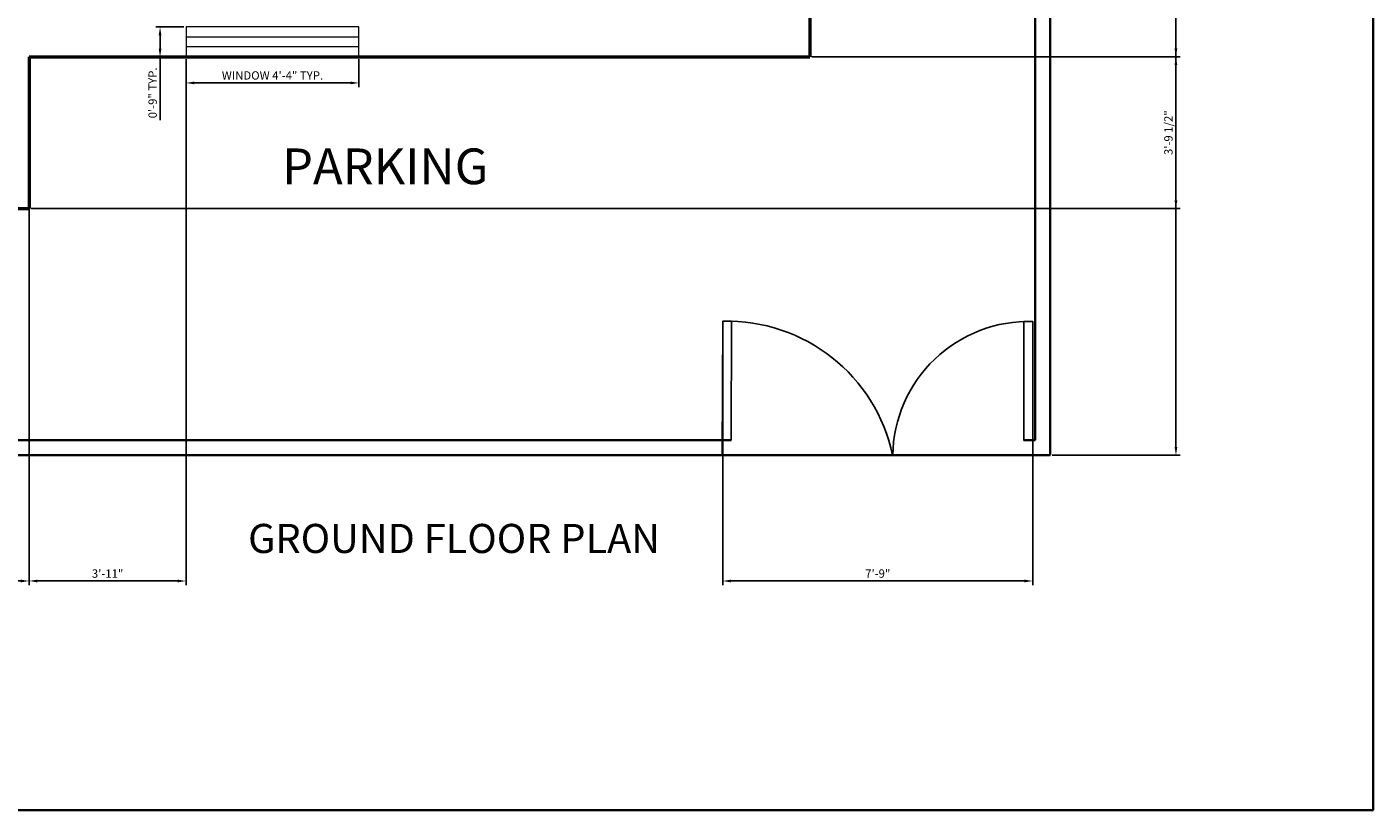
# Model space of a CAD drawing. Units: inches. Extents: x 65 to 818, y -87 to 880.
# Tile 3 of 6: x 414 to 818, y -87 to 148. Entities that reach past the tile are written whole.
import ezdxf

# ---------------------------------------------------------------- set-up
doc = ezdxf.new("R2010")
doc.units = ezdxf.units.IN
for name, color, linetype, lineweight in [('A-ANNO-DIMS', 2, 'Continuous', 18), ('A-ANNO-TEXT', 7, 'Continuous', 25), ('A-ANNO-TTLB', 7, 'Continuous', 35), ('A-AREA-IDEN', 7, 'Continuous', 25), ('A-GLAZ', 4, 'Continuous', 18), ('A-WALL', 7, 'Continuous', 50), ('C-PROP', 7, 'Continuous', 35), ('L-SITE-GATE', 3, 'Continuous', 25)]:
    doc.layers.add(name, color=color, linetype=linetype, lineweight=lineweight)
doc.styles.get("Standard").update_dxf_attribs({"font": 'arial.ttf'})
doc.dimstyles.new('ISO-25', dxfattribs={"dimtxt": 2.5, "dimasz": 2.5, "dimexe": 1.25, "dimexo": 0.625, "dimtad": 1, "dimtxsty": 'Standard', "dimcen": 2.5, "dimadec": 0, "dimazin": 0, "dimtfac": 1, "dimtmove": 0, "dimatfit": 3, "dimfxl": 1, "dimarcsym": 0})

# ---------------------------------------------------------------- blocks, each defined once
blk = doc.blocks.new('WIN-52X9-PLAN')
for p, q in [((9, 51.82), (0, 51.82)), ((0, 51.82), (0, 0)), ((3, 0), (3, 51.82)), ((6, 51.82), (6, 0)), ((9, 0), (9, 51.82)), ((0, 0), (9, 0))]:
    blk.add_line(p, q)
blk = doc.blocks.new('*D24')
at = {"layer": 'A-ANNO-DIMS', "color": 0, "lineweight": -2, "transparency": 16777216}
for p, q in [((461.82, 137.86), (461.82, 129.46)), ((513.64, 137.86), (513.64, 129.46)), ((464.32, 130.71), (511.14, 130.71))]:
    blk.add_line(p, q, dxfattribs=at)
at = {"layer": 'A-ANNO-DIMS', "color": 0, "transparency": 16777216}
for points in [[(464.32, 131.13), (464.32, 130.3), (461.82, 130.71)], [(511.14, 131.13), (511.14, 130.3), (513.64, 130.71)]]:
    blk.add_solid(points, dxfattribs=at)
at = {"layer": 'Defpoints', "color": 0, "transparency": 16777216}
for p in [(461.82, 138.49), (513.64, 138.49), (513.64, 130.71)]:
    blk.add_point(p, dxfattribs=at)
at = {"layer": 'A-ANNO-DIMS', "color": 0, "transparency": 16777216, "insert": (487.73, 132.63), "char_height": 2.5, "attachment_point": 5}
blk.add_mtext('WINDOW 4\'-4" TYP.', dxfattribs=at)
blk = doc.blocks.new('*D25')
at = {"layer": 'A-ANNO-DIMS', "color": 0, "lineweight": -2, "transparency": 16777216}
for p, q in [((461.19, 147.49), (452.79, 147.49)), ((454.04, 144.99), (454.04, 140.99)), ((461.19, 138.49), (452.79, 138.49)), ((454.04, 138.49), (454.04, 119.5))]:
    blk.add_line(p, q, dxfattribs=at)
at = {"layer": 'A-ANNO-DIMS', "color": 0, "transparency": 16777216}
for points in [[(453.63, 144.99), (454.46, 144.99), (454.04, 147.49)], [(453.63, 140.99), (454.46, 140.99), (454.04, 138.49)]]:
    blk.add_solid(points, dxfattribs=at)
at = {"layer": 'Defpoints', "color": 0, "transparency": 16777216}
for p in [(461.82, 147.49), (454.04, 138.49), (461.82, 138.49)]:
    blk.add_point(p, dxfattribs=at)
at = {"layer": 'A-ANNO-DIMS', "color": 0, "transparency": 16777216, "insert": (452.14, 127.74), "char_height": 2.5, "attachment_point": 5, "rotation": 90}
blk.add_mtext('0\'-9" TYP.', dxfattribs=at)
blk = doc.blocks.new('*D54')
at = {"layer": 'A-ANNO-DIMS', "color": 0, "lineweight": -2, "transparency": 16777216}
for p, q in [((649.42, 138.54), (759.75, 138.54)), ((758.5, 95.54), (758.5, 136.04)), ((415.42, 93.04), (759.75, 93.04))]:
    blk.add_line(p, q, dxfattribs=at)
at = {"layer": 'A-ANNO-DIMS', "color": 0, "transparency": 16777216}
for points in [[(758.08, 136.04), (758.92, 136.04), (758.5, 138.54)], [(758.08, 95.54), (758.92, 95.54), (758.5, 93.04)]]:
    blk.add_solid(points, dxfattribs=at)
at = {"layer": 'Defpoints', "color": 0, "transparency": 16777216}
for p in [(648.8, 138.54), (758.5, 138.54), (414.8, 93.04)]:
    blk.add_point(p, dxfattribs=at)
at = {"layer": 'A-ANNO-DIMS', "color": 0, "transparency": 16777216, "insert": (756.58, 115.79), "char_height": 2.5, "attachment_point": 5, "rotation": 90}
blk.add_mtext('3\'-9 1/2"', dxfattribs=at)
blk = doc.blocks.new('*D57')
at = {"layer": 'A-ANNO-DIMS', "color": 0, "lineweight": -2, "transparency": 16777216}
for p, q in [((622.67, 58.62), (622.67, -19.91)), ((715.59, 58.54), (715.59, -19.91)), ((625.17, -18.66), (713.09, -18.66))]:
    blk.add_line(p, q, dxfattribs=at)
at = {"layer": 'A-ANNO-DIMS', "color": 0, "transparency": 16777216}
for points in [[(625.17, -18.25), (625.17, -19.08), (622.67, -18.66)], [(713.09, -18.25), (713.09, -19.08), (715.59, -18.66)]]:
    blk.add_solid(points, dxfattribs=at)
at = {"layer": 'Defpoints', "color": 0, "transparency": 16777216}
for p in [(622.67, 59.25), (715.59, 59.17), (715.59, -18.66)]:
    blk.add_point(p, dxfattribs=at)
at = {"layer": 'A-ANNO-DIMS', "color": 0, "transparency": 16777216, "insert": (669.13, -16.76), "char_height": 2.5, "attachment_point": 5}
blk.add_mtext('7\'-9"', dxfattribs=at)
blk = doc.blocks.new('*D60')
at = {"layer": 'A-ANNO-DIMS', "color": 0, "lineweight": -2, "transparency": 16777216}
for p, q in [((649.42, 376.08), (759.75, 376.08)), ((758.5, 141.04), (758.5, 373.58)), ((649.42, 138.54), (759.75, 138.54))]:
    blk.add_line(p, q, dxfattribs=at)
at = {"layer": 'A-ANNO-DIMS', "color": 0, "transparency": 16777216}
for points in [[(758.08, 373.58), (758.92, 373.58), (758.5, 376.08)], [(758.08, 141.04), (758.92, 141.04), (758.5, 138.54)]]:
    blk.add_solid(points, dxfattribs=at)
at = {"layer": 'Defpoints', "color": 0, "transparency": 16777216}
for p in [(648.8, 376.08), (758.5, 376.08), (648.8, 138.54)]:
    blk.add_point(p, dxfattribs=at)
at = {"layer": 'A-ANNO-DIMS', "color": 0, "transparency": 16777216, "insert": (756.58, 257.31), "char_height": 2.5, "attachment_point": 5, "rotation": 90}
blk.add_mtext('19\'-9 1/2"', dxfattribs=at)
blk = doc.blocks.new('*D64')
at = {"layer": 'A-ANNO-DIMS', "color": 0, "lineweight": -2, "transparency": 16777216}
for p, q in [((414.8, 137.92), (414.8, -19.91)), ((461.82, 137.86), (461.82, -19.91)), ((417.3, -18.66), (459.32, -18.66))]:
    blk.add_line(p, q, dxfattribs=at)
at = {"layer": 'A-ANNO-DIMS', "color": 0, "transparency": 16777216}
for points in [[(417.3, -18.25), (417.3, -19.08), (414.8, -18.66)], [(459.32, -18.25), (459.32, -19.08), (461.82, -18.66)]]:
    blk.add_solid(points, dxfattribs=at)
at = {"layer": 'Defpoints', "color": 0, "transparency": 16777216}
for p in [(414.8, 138.54), (461.82, 138.49), (461.82, -18.66)]:
    blk.add_point(p, dxfattribs=at)
at = {"layer": 'A-ANNO-DIMS', "color": 0, "transparency": 16777216, "insert": (438.31, -16.76), "char_height": 2.5, "attachment_point": 5}
blk.add_mtext('3\'-11"', dxfattribs=at)
blk = doc.blocks.new('*D65')
at = {"layer": 'A-ANNO-DIMS', "color": 0, "lineweight": -2, "transparency": 16777216}
for p, q in [((721.42, 363.55), (759.75, 363.55)), ((758.5, 21.54), (758.5, 361.05)), ((721.42, 19.04), (759.75, 19.04))]:
    blk.add_line(p, q, dxfattribs=at)
at = {"layer": 'A-ANNO-DIMS', "color": 0, "transparency": 16777216}
for points in [[(758.08, 361.05), (758.92, 361.05), (758.5, 363.55)], [(758.08, 21.54), (758.92, 21.54), (758.5, 19.04)]]:
    blk.add_solid(points, dxfattribs=at)
at = {"layer": 'Defpoints', "color": 0, "transparency": 16777216}
for p in [(720.8, 363.55), (758.5, 363.55), (720.8, 19.04)]:
    blk.add_point(p, dxfattribs=at)
at = {"layer": 'A-ANNO-DIMS', "color": 0, "transparency": 16777216, "insert": (756.58, 191.3), "char_height": 2.5, "attachment_point": 5, "rotation": 90}
blk.add_mtext('28\'-8 1/2"', dxfattribs=at)
blk = doc.blocks.new('*D71')
at = {"layer": 'A-ANNO-DIMS', "color": 0, "lineweight": -2, "transparency": 16777216}
for p, q in [((414.8, 92.42), (414.8, -19.91)), ((240.8, 18.42), (240.8, -19.91)), ((243.3, -18.66), (412.3, -18.66))]:
    blk.add_line(p, q, dxfattribs=at)
at = {"layer": 'A-ANNO-DIMS', "color": 0, "transparency": 16777216}
for points in [[(243.3, -18.25), (243.3, -19.08), (240.8, -18.66)], [(412.3, -18.25), (412.3, -19.08), (414.8, -18.66)]]:
    blk.add_solid(points, dxfattribs=at)
at = {"layer": 'Defpoints', "color": 0, "transparency": 16777216}
for p in [(414.8, 93.04), (240.8, 19.04), (414.8, -18.66)]:
    blk.add_point(p, dxfattribs=at)
at = {"layer": 'A-ANNO-DIMS', "color": 0, "transparency": 16777216, "insert": (327.8, -16.76), "char_height": 2.5, "attachment_point": 5}
blk.add_mtext('14\'-6"', dxfattribs=at)

msp = doc.modelspace()

# ---------------------------------------------------------------- linework, layer by layer
at = {"layer": 'A-ANNO-TTLB'}
msp.add_lwpolyline([(64.55, 880.46), (817.59, 880.46), (817.59, -87.37), (64.55, -87.37)], close=True, dxfattribs=at)
at = {"layer": 'A-WALL'}
for p, q in [((648.8, 703.04), (648.8, 138.54)), ((414.8, 138.54), (648.8, 138.54)), ((414.8, 138.54), (414.8, 93.04)), ((249.8, 93.04), (414.8, 93.04))]:
    msp.add_line(p, q, dxfattribs=at)
at = {"layer": 'C-PROP'}
for p, q in [((716.3, 734.54), (716.3, 23.54)), ((720.8, 366.22), (720.8, 19.04)), ((625.16, 23.54), (249.8, 23.54)), ((716.3, 23.54), (712.92, 23.54)), ((720.8, 19.04), (240.8, 19.04))]:
    msp.add_line(p, q, dxfattribs=at)
at = {"layer": 'L-SITE-GATE'}
msp.add_lwpolyline([(625.16, 23.54), (625.34, 59.25), (622.67, 59.25), (622.47, 19.04)], dxfattribs=at)
msp.add_lwpolyline([(712.9, 23.5), (715.57, 23.5), (715.59, 59.17), (712.92, 59.17)], close=True, dxfattribs=at)
for centre, radius, start, end in [((624, 8.57), 50.69, 11.911, 91.511), ((714.4, 18.41), 40.78, 88.3321, 179.1109)]:
    msp.add_arc(centre, radius, start, end, dxfattribs=at)

# ---------------------------------------------------------------- block references
at = {"layer": 'A-GLAZ', "rotation": 269.9999999999999}
msp.add_blockref('WIN-52X9-PLAN', (461.82, 147.49), dxfattribs=at)

# ---------------------------------------------------------------- texts
at = {"layer": 'A-ANNO-TEXT', "insert": (480.42, -1.54), "char_height": 8.7281, "attachment_point": 1}
msp.add_mtext_dynamic_manual_height_columns('GROUND FLOOR PLAN ', width=274.3156, gutter_width=43.64, heights=[0], dxfattribs=at)
at = {"layer": 'A-AREA-IDEN', "insert": (490.62, 111.06), "char_height": 10.719, "attachment_point": 1}
msp.add_mtext_dynamic_manual_height_columns('PARKING', width=326.6484, gutter_width=53.59, heights=[0], dxfattribs=at)

# ---------------------------------------------------------------- dimensions: what is measured, and where the dimension line sits
at = {"layer": 'A-ANNO-DIMS'}
for base, p1, p2, picture, middle in [((758.5, 376.08), (648.8, 138.54), (648.8, 376.08), '*D60', (756.58, 257.31)), ((758.5, 363.55), (720.8, 19.04), (720.8, 363.55), '*D65', (756.58, 191.3)), ((758.5, 138.54), (414.8, 93.04), (648.8, 138.54), '*D54', (756.58, 115.79))]:
    dim = msp.add_linear_dim(base=base, p1=p1, p2=p2, angle=90, dimstyle='ISO-25', override={"dimdec": 1, "dimlfac": 1, "dimrnd": 0, "dimzin": 1, "dimdsep": 46, "dimlunit": 4, "dimfrac": 2}, dxfattribs=at)
    dim.commit()
    dim.dimension.update_dxf_attribs({"geometry": picture, "text_midpoint": middle})
dim = msp.add_linear_dim(base=(454.04, 138.49), p1=(461.82, 147.49), p2=(461.82, 138.49), angle=270, text='<> TYP.', dimstyle='ISO-25', override={"dimdec": 1, "dimlfac": 1, "dimrnd": 0, "dimzin": 1, "dimdsep": 46, "dimlunit": 4, "dimfrac": 2}, dxfattribs=at)
dim.commit()
dim.dimension.update_dxf_attribs({"geometry": '*D25', "text_midpoint": (452.14, 127.74)})
for base, p1, p2, picture, middle in [((461.82, -18.66), (414.8, 138.54), (461.82, 138.49), '*D64', (438.31, -16.76)), ((414.8, -18.66), (240.8, 19.04), (414.8, 93.04), '*D71', (327.8, -16.76)), ((715.59, -18.66), (622.67, 59.25), (715.59, 59.17), '*D57', (669.13, -16.76))]:
    dim = msp.add_linear_dim(base=base, p1=p1, p2=p2, dimstyle='ISO-25', override={"dimdec": 1, "dimlfac": 1, "dimrnd": 0, "dimzin": 1, "dimdsep": 46, "dimlunit": 4, "dimfrac": 2}, dxfattribs=at)
    dim.commit()
    dim.dimension.update_dxf_attribs({"geometry": picture, "text_midpoint": middle})
dim = msp.add_linear_dim(base=(513.64, 130.71), p1=(461.82, 138.49), p2=(513.64, 138.49), text='WINDOW <> TYP.', dimstyle='ISO-25', override={"dimdec": 1, "dimlfac": 1, "dimrnd": 0, "dimzin": 1, "dimdsep": 46, "dimlunit": 4, "dimfrac": 2}, dxfattribs=at)
dim.commit()
dim.dimension.update_dxf_attribs({"geometry": '*D24', "text_midpoint": (487.73, 132.63)})

doc.saveas('drawing.dxf')
